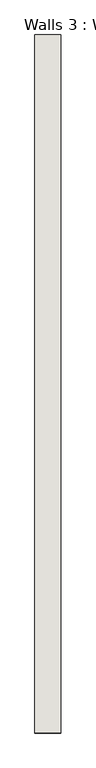
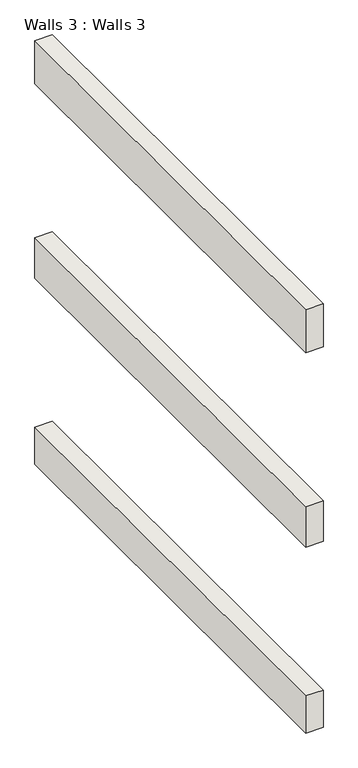
"""IFC4 building model written with IfcOpenShell, lengths in millimetres: wall geometry, Walls 3 : Walls 3."""

from ifc_helpers import new_model, si_unit, frame, origin, place, context, project, spatial, polyline, outline, extrude, source, transform, mapped, element, save


def walls_3_walls_3_273bb310(model_context):
    return source(origin(), model_context, "Body", "SweptSolid", [
        extrude(outline(polyline([(-3084.5864811, 10958.2297737), (-3084.5864811, 2754.0297737), (-3389.3864811, 2754.0297737), (-3389.3864811, 10958.2297737), (-3084.5864811, 10958.2297737)])), frame((0.0, 0.0, 7315.2), z_axis=(0.0, 0.0, 1.0), x_axis=(1.0, 0.0, 0.0)), (0.0, 0.0, 1.0), 686.3630935),
        extrude(outline(polyline([(-3084.5864811, 10958.2297737), (-3084.5864811, 2754.0297737), (-3389.3864811, 2754.0297737), (-3389.3864811, 10958.2297737), (-3084.5864811, 10958.2297737)])), frame((0.0, 0.0, 10755.6862551), z_axis=(0.0, 0.0, 1.0), x_axis=(1.0, 0.0, 0.0)), (0.0, 0.0, 1.0), 749.7320941),
        extrude(outline(polyline([(-3084.5864811, 10958.2297737), (-3084.5864811, 2754.0297737), (-3389.3864811, 2754.0297737), (-3389.3864811, 10958.2297737), (-3084.5864811, 10958.2297737)])), frame((0.0, 0.0, 14349.977535), z_axis=(0.0, 0.0, 1.0), x_axis=(1.0, 0.0, 0.0)), (0.0, 0.0, 1.0), 797.4209956),
    ])


if __name__ == "__main__":
    model = new_model("IFC4")
    model_context = context("Model", 3, world=origin())
    ifc_project = project(units=[si_unit("LENGTHUNIT", "METRE", prefix="MILLI")], contexts=[model_context])
    site = spatial("IfcSite", under=ifc_project)
    building = spatial("IfcBuilding", under=site)
    placement = place(None, origin())
    walls_3_walls_3_shape = walls_3_walls_3_273bb310(model_context)
    element("IfcWall", 1, ObjectType="Walls 3 : Walls 3", at=placement, inside=building, context=model_context, shape_type="MappedRepresentation", body=[
        mapped(walls_3_walls_3_shape, transform((0.0, 0.0, 0.0), x_axis=(1.0, 0.0, 0.0), y_axis=(0.0, 1.0, 0.0), z_axis=(0.0, 0.0, 1.0))),
    ])
    save(model, "model.ifc")

# Revit data of these elements
# Element 1 (IfcWall, "Walls 3 : Walls 3")
#   Materials on its faces: "Default Wall"
# Materials
#   "Default Wall": colour RGB 128 128 128, transparency 0
